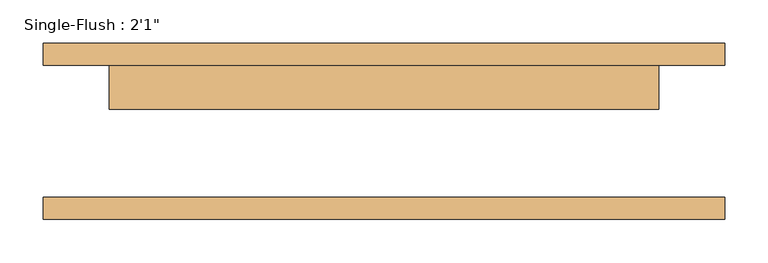
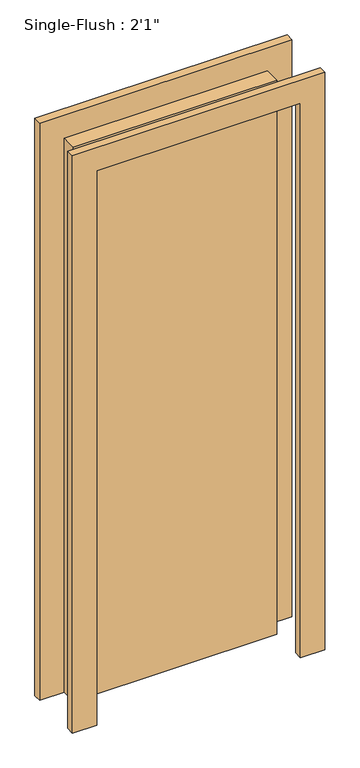
"""IFC4 building model written with IfcOpenShell, lengths in millimetres: door geometry."""

from ifc_helpers import new_model, si_unit, frame, origin, origin_with_axes, place, context, project, spatial, polyline, outline, extrude, source, transform, mapped, element, save


def door_57c759c4(model_context):
    return source(origin(), model_context, "Body", "SweptSolid", [
        extrude(outline(polyline([(1905.0, -393.7), (0.0, -393.7), (0.0, -317.5), (1828.8, -317.5), (1828.8, 317.5), (0.0, 317.5), (0.0, 393.7), (1905.0, 393.7), (1905.0, -393.7)])), frame((0.0, 76.2, 0.0), z_axis=(0.0, 1.0, 0.0), x_axis=(0.0, 0.0, 1.0)), (0.0, 0.0, 1.0), 25.4),
        extrude(outline(polyline([(1905.0, 393.7), (1905.0, -393.7), (0.0, -393.7), (0.0, -317.5), (1828.8, -317.5), (1828.8, 317.5), (0.0, 317.5), (0.0, 393.7), (1905.0, 393.7)])), frame((0.0, -101.6, 0.0), z_axis=(0.0, 1.0, 0.0), x_axis=(0.0, 0.0, 1.0)), (0.0, 0.0, 1.0), 25.4),
        extrude(outline(polyline([(317.5, 25.4), (-317.5, 25.4), (-317.5, 76.2), (317.5, 76.2), (317.5, 25.4)])), origin_with_axes(), (0.0, 0.0, 1.0), 1828.8),
    ])


if __name__ == "__main__":
    model = new_model("IFC4")
    model_context = context("Model", 3, world=origin())
    ifc_project = project(units=[si_unit("LENGTHUNIT", "METRE", prefix="MILLI")], contexts=[model_context])
    site = spatial("IfcSite", under=ifc_project)
    building = spatial("IfcBuilding", under=site)
    placement = place(None, origin())
    door_shape = door_57c759c4(model_context)
    element("IfcDoor", 1, ObjectType="Single-Flush : 2'1\"", at=placement, inside=building, context=model_context, shape_type="MappedRepresentation", body=[
        mapped(door_shape, transform((0.0, 0.0, 0.0), x_axis=(1.0, 0.0, 0.0), y_axis=(0.0, 1.0, 0.0), z_axis=(0.0, 0.0, 1.0))),
    ])
    save(model, "model.ifc")

# Revit data of these elements
# Type "Single-Flush : 2'1\""
#   Type Mark = "9"
#   Construction Type Id = "MDOOR"
#   Assembly Code = "C1020"
#   Analytic Construction = "Metal"
#   Thickness = 0' - 2"
#   Heat Transfer Coefficient (U) = 0.651978 BTU/(h·ft²·°F)
#   Height = 6' - 0"
#   Trim Projection Ext = 0' - 1"
#   Trim Projection Int = 0' - 1"
#   Trim Width = 0' - 3"
#   Width = 2' - 1"
#   Define Thermal Properties by = 1
#   Door Material = Door - Panel
#   Frame Material = Door - Frame
#   Visual Light Transmittance = 0
#   Solar Heat Gain Coefficient = 0
#   Function = (empty or 0)
#   Wall Closure = (empty or 0)
# Element 1 (IfcDoor, "Single-Flush : 2'1\"")
#   Materials on its faces: "Door - Frame", "Door - Panel"
# Materials
#   "Door - Panel": class "Wood", colour RGB 210 159 95, transparency 0, Cost = 0
#   "Door - Frame": colour RGB 118 70 51, transparency 0, Cost = 0
